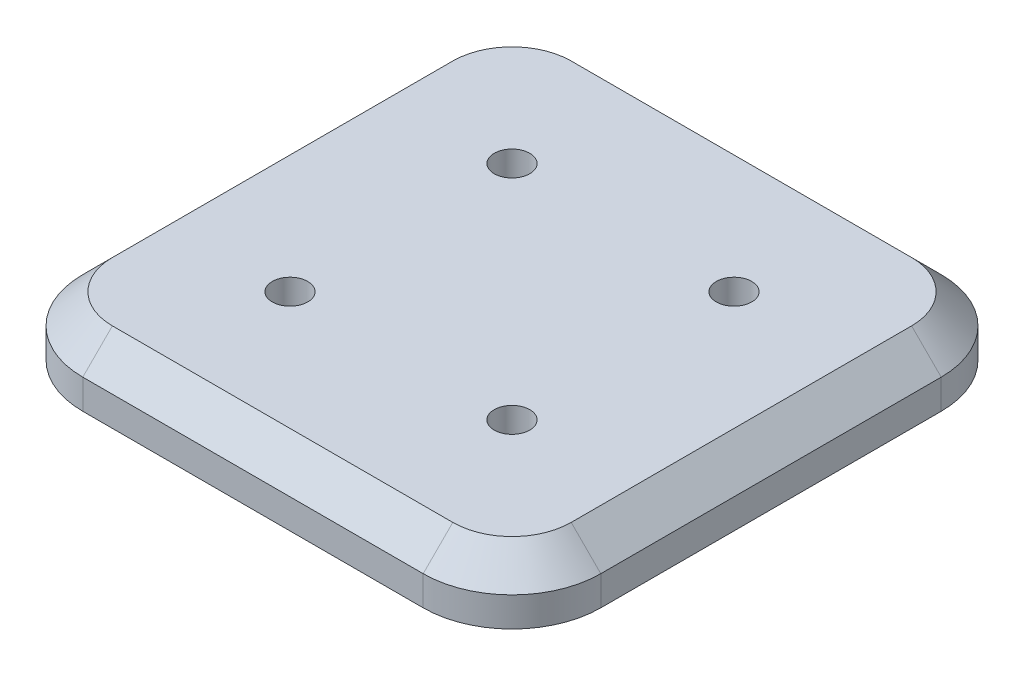
from build123d import *

# Parameters (mm, degrees)
BASE_PLATE_SKETCH_175X175_W = 175
BASE_PLATE_SKETCH_175X175_H = 175
BASE_PLATE_DEPTH            = 20
CORNER_FILLETS_R30_R        = 30
EDGE_CHAMFER_10X45_SIZE     = 10
DOWEL_HOLES_12_INNER_D      = 12
DOWEL_HOLES_12_INNER_DEPTH  = 10
DOWEL_HOLES_12_INNER_TIP    = 3.605163714
DOWEL_HOLES_12_OUTER_D      = 12
DOWEL_HOLES_12_OUTER_DEPTH  = 10
DOWEL_HOLES_12_OUTER_TIP    = 3.605163714


with BuildPart() as part:
    # Base Plate Sketch 175x175 → Base Plate (new body)
    with BuildSketch(Plane(origin=(0, 0, 0), x_dir=(1, 0, 0), z_dir=(0, 1, 0))):
        Rectangle(BASE_PLATE_SKETCH_175X175_W, BASE_PLATE_SKETCH_175X175_H)
    extrude(amount=BASE_PLATE_DEPTH)

    # Corner Fillets R30
    corner_fillets_r30_edges = [part.edges().sort_by_distance(p)[0] for p in [
        (87.5, 10, 87.5),
        (-87.5, 10, 87.5),
        (-87.5, 10, -87.5),
        (87.5, 10, -87.5),
    ]]
    fillet(corner_fillets_r30_edges, radius=CORNER_FILLETS_R30_R)

    # Edge Chamfer 10x45
    edge_chamfer_10x45_edges = [part.edges().sort_by_distance(p)[0] for p in [
        (-87.5, 20, 0),
        (0, 20, -87.5),
        (87.5, 20, 0),
        (0, 20, 87.5),
        (-78.713203436, 20, 78.713203436),
        (78.713203436, 20, 78.713203436),
        (78.713203436, 20, -78.713203436),
        (-78.713203436, 20, -78.713203436),
    ]]
    chamfer(edge_chamfer_10x45_edges, length=EDGE_CHAMFER_10X45_SIZE)

    # Dowel Holes Ø12 Inner
    with Locations(Plane(origin=(-37.5, 20, -37.5), x_dir=(0, 0, 1), z_dir=(0, 1, 0))):
        with Locations((0, 0), (0, 75), (75, 75), (75, 0)):
            Hole(DOWEL_HOLES_12_INNER_D / 2, depth=DOWEL_HOLES_12_INNER_DEPTH)
            with Locations((0, 0, -(DOWEL_HOLES_12_INNER_DEPTH + DOWEL_HOLES_12_INNER_TIP / 2))):  # 118° drill point
                Cone(0, DOWEL_HOLES_12_INNER_D / 2, DOWEL_HOLES_12_INNER_TIP, mode=Mode.SUBTRACT)

    # Dowel Holes Ø12 Outer
    with Locations(Plane(origin=(-62.5, 0, 62.5), x_dir=(0, 0, -1), z_dir=(0, -1, 0))):
        with Locations((0, 0), (0, 125), (125, 125), (125, 0)):
            Hole(DOWEL_HOLES_12_OUTER_D / 2, depth=DOWEL_HOLES_12_OUTER_DEPTH)
            with Locations((0, 0, -(DOWEL_HOLES_12_OUTER_DEPTH + DOWEL_HOLES_12_OUTER_TIP / 2))):  # 118° drill point
                Cone(0, DOWEL_HOLES_12_OUTER_D / 2, DOWEL_HOLES_12_OUTER_TIP, mode=Mode.SUBTRACT)


solid = part.part
